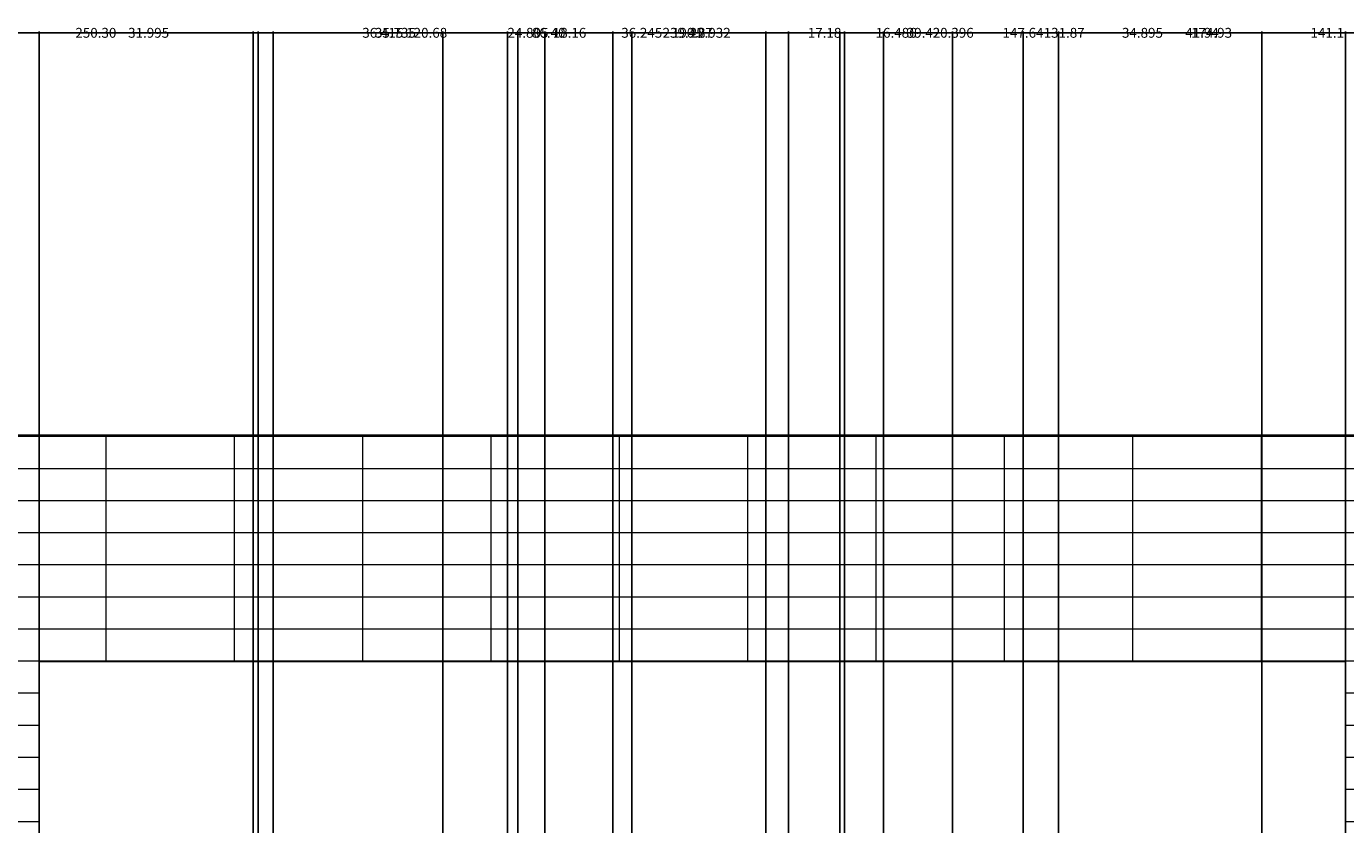
# Model space of a CAD drawing. Units: inches. Extents: x 241 to 943, y 109 to 1396.
# Tile 32 of 34: x 532 to 725, y 1279 to 1396. Entities that reach past the tile are written whole.
import ezdxf

# ---------------------------------------------------------------- set-up
doc = ezdxf.new("R2010")
doc.units = ezdxf.units.IN
doc.header["$MEASUREMENT"] = 0
for name, color, linetype, lineweight in [('A-ANNO-DIMS', 2, 'Continuous', 18), ('A-ELEV', 7, 'Continuous', 25), ('A-GLAZ', 4, 'Continuous', 18), ('A-WALL-PATT', 8, 'Continuous', 13)]:
    doc.layers.add(name, color=color, linetype=linetype, lineweight=lineweight)
doc.styles.get("Standard").update_dxf_attribs({"font": 'arial.ttf'})
doc.dimstyles.get("Standard").update_dxf_attribs({"dimtxt": 1.4375, "dimasz": 0.18, "dimexe": 0.18, "dimexo": 0.0625, "dimgap": 0.09, "dimtad": 0, "dimtih": 1, "dimtoh": 1, "dimdec": 4, "dimzin": 0, "dimdsep": 46, "dimlunit": 4, "dimtxsty": 'Standard', "dimcen": 0.09, "dimadec": 0, "dimazin": 0, "dimtfac": 1, "dimtdec": 4, "dimtofl": 0, "dimtmove": 0, "dimatfit": 3, "dimfxl": 1, "dimtolj": 1, "dimtzin": 0, "dimarcsym": 0})

# ---------------------------------------------------------------- blocks, each defined once
blk = doc.blocks.new('*D12')
at = {"layer": 'A-ANNO-DIMS', "color": 0, "lineweight": -2, "transparency": 16777216}
for p, q in [((530.23, 384.24), (530.23, 1395.05)), ((530.41, 1394.87), (587.56, 1394.87)), ((650.73, 1394.87), (593.58, 1394.87)), ((650.91, 384.24), (650.91, 1395.05))]:
    blk.add_line(p, q, dxfattribs=at)
at = {"layer": 'A-ANNO-DIMS', "color": 0, "transparency": 16777216}
for points in [[(530.41, 1394.9), (530.41, 1394.84), (530.23, 1394.87)], [(650.73, 1394.9), (650.73, 1394.84), (650.91, 1394.87)]]:
    blk.add_solid(points, dxfattribs=at)
at = {"layer": 'Defpoints', "color": 0, "transparency": 16777216}
for p in [(650.91, 1394.87), (530.23, 384.18), (650.91, 384.18)]:
    blk.add_point(p, dxfattribs=at)
at = {"layer": 'A-ANNO-DIMS', "color": 0, "transparency": 16777216, "insert": (590.57, 1394.87), "char_height": 1.438, "attachment_point": 5}
blk.add_mtext('\\A1;120.68', dxfattribs=at)
blk = doc.blocks.new('*D13')
at = {"layer": 'A-ANNO-DIMS', "color": 0, "lineweight": -2, "transparency": 16777216}
for p, q in [((650.91, 384.24), (650.91, 1395.05)), ((651.09, 1394.87), (656.14, 1394.87)), ((667.21, 1394.87), (662.16, 1394.87)), ((667.39, 290.06), (667.39, 1395.05))]:
    blk.add_line(p, q, dxfattribs=at)
at = {"layer": 'A-ANNO-DIMS', "color": 0, "transparency": 16777216}
for points in [[(651.09, 1394.9), (651.09, 1394.84), (650.91, 1394.87)], [(667.21, 1394.9), (667.21, 1394.84), (667.39, 1394.87)]]:
    blk.add_solid(points, dxfattribs=at)
at = {"layer": 'Defpoints', "color": 0, "transparency": 16777216}
for p in [(667.39, 1394.87), (650.91, 384.18), (667.39, 290)]:
    blk.add_point(p, dxfattribs=at)
at = {"layer": 'A-ANNO-DIMS', "color": 0, "transparency": 16777216, "insert": (659.15, 1394.87), "char_height": 1.438, "attachment_point": 5}
blk.add_mtext('\\A1;16.486', dxfattribs=at)
blk = doc.blocks.new('*D14')
at = {"layer": 'A-ANNO-DIMS', "color": 0, "lineweight": -2, "transparency": 16777216}
for p, q in [((667.39, 290.06), (667.39, 1395.05)), ((667.57, 1394.87), (727.7, 1394.87)), ((793.85, 1394.87), (733.72, 1394.87)), ((794.03, 290.06), (794.03, 1395.05))]:
    blk.add_line(p, q, dxfattribs=at)
at = {"layer": 'A-ANNO-DIMS', "color": 0, "transparency": 16777216}
for points in [[(667.57, 1394.9), (667.57, 1394.84), (667.39, 1394.87)], [(793.85, 1394.9), (793.85, 1394.84), (794.03, 1394.87)]]:
    blk.add_solid(points, dxfattribs=at)
at = {"layer": 'Defpoints', "color": 0, "transparency": 16777216}
for p in [(794.03, 1394.87), (667.39, 290), (794.03, 290)]:
    blk.add_point(p, dxfattribs=at)
at = {"layer": 'A-ANNO-DIMS', "color": 0, "transparency": 16777216, "insert": (730.71, 1394.87), "char_height": 1.438, "attachment_point": 5}
blk.add_mtext('\\A1;126.63', dxfattribs=at)
blk = doc.blocks.new('*D18')
at = {"layer": 'A-ANNO-DIMS', "color": 0, "lineweight": -2, "transparency": 16777216}
for p, q in [((508.31, 1336.18), (508.31, 1395.05)), ((508.49, 1394.87), (624.94, 1394.87)), ((747.58, 1394.87), (631.12, 1394.87)), ((747.76, 1336.18), (747.76, 1395.05))]:
    blk.add_line(p, q, dxfattribs=at)
at = {"layer": 'A-ANNO-DIMS', "color": 0, "transparency": 16777216}
for points in [[(508.49, 1394.9), (508.49, 1394.84), (508.31, 1394.87)], [(747.58, 1394.9), (747.58, 1394.84), (747.76, 1394.87)]]:
    blk.add_solid(points, dxfattribs=at)
at = {"layer": 'Defpoints', "color": 0, "transparency": 16777216}
for p in [(747.76, 1394.87), (508.31, 1336.12), (747.76, 1336.12)]:
    blk.add_point(p, dxfattribs=at)
at = {"layer": 'A-ANNO-DIMS', "color": 0, "transparency": 16777216, "insert": (628.03, 1394.87), "char_height": 1.438, "attachment_point": 5}
blk.add_mtext('\\A1;239.45', dxfattribs=at)
blk = doc.blocks.new('*D56')
at = {"layer": 'A-ANNO-DIMS', "color": 0, "lineweight": -2, "transparency": 16777216}
for p, q in [((533.95, 1303.09), (533.95, 1395.05)), ((534.13, 1394.87), (626.38, 1394.87)), ((724.64, 1394.87), (632.39, 1394.87)), ((724.82, 1303.09), (724.82, 1395.05))]:
    blk.add_line(p, q, dxfattribs=at)
at = {"layer": 'A-ANNO-DIMS', "color": 0, "transparency": 16777216}
for points in [[(534.13, 1394.9), (534.13, 1394.84), (533.95, 1394.87)], [(724.64, 1394.9), (724.64, 1394.84), (724.82, 1394.87)]]:
    blk.add_solid(points, dxfattribs=at)
at = {"layer": 'Defpoints', "color": 0, "transparency": 16777216}
for p in [(724.82, 1394.87), (533.95, 1303.03), (724.82, 1303.03)]:
    blk.add_point(p, dxfattribs=at)
at = {"layer": 'A-ANNO-DIMS', "color": 0, "transparency": 16777216, "insert": (629.39, 1394.87), "char_height": 1.438, "attachment_point": 5}
blk.add_mtext('\\A1;190.87', dxfattribs=at)
blk = doc.blocks.new('*D57')
at = {"layer": 'A-ANNO-DIMS', "color": 0, "lineweight": -2, "transparency": 16777216}
for p, q in [((508.31, 1070.92), (508.31, 1395.05)), ((508.49, 1394.87), (518.04, 1394.87)), ((533.77, 1394.87), (524.21, 1394.87)), ((533.95, 1108.23), (533.95, 1395.05))]:
    blk.add_line(p, q, dxfattribs=at)
at = {"layer": 'A-ANNO-DIMS', "color": 0, "transparency": 16777216}
for points in [[(508.49, 1394.9), (508.49, 1394.84), (508.31, 1394.87)], [(533.77, 1394.9), (533.77, 1394.84), (533.95, 1394.87)]]:
    blk.add_solid(points, dxfattribs=at)
at = {"layer": 'Defpoints', "color": 0, "transparency": 16777216}
for p in [(533.95, 1394.87), (533.95, 1108.17), (508.31, 1070.85)]:
    blk.add_point(p, dxfattribs=at)
at = {"layer": 'A-ANNO-DIMS', "color": 0, "transparency": 16777216, "insert": (521.13, 1394.87), "char_height": 1.438, "attachment_point": 5}
blk.add_mtext('\\A1;25.646', dxfattribs=at)
blk = doc.blocks.new('*D62')
at = {"layer": 'A-ANNO-DIMS', "color": 0, "lineweight": -2, "transparency": 16777216}
for p, q in [((424.11, 568.89), (424.11, 1395.05)), ((424.29, 1394.87), (492.35, 1394.87)), ((565.02, 1394.87), (496.96, 1394.87)), ((565.2, 568.89), (565.2, 1395.05))]:
    blk.add_line(p, q, dxfattribs=at)
at = {"layer": 'A-ANNO-DIMS', "color": 0, "transparency": 16777216}
for points in [[(424.29, 1394.9), (424.29, 1394.84), (424.11, 1394.87)], [(565.02, 1394.9), (565.02, 1394.84), (565.2, 1394.87)]]:
    blk.add_solid(points, dxfattribs=at)
at = {"layer": 'Defpoints', "color": 0, "transparency": 16777216}
for p in [(565.2, 1394.87), (424.11, 568.83), (565.2, 568.83)]:
    blk.add_point(p, dxfattribs=at)
at = {"layer": 'A-ANNO-DIMS', "color": 0, "transparency": 16777216, "insert": (494.66, 1394.87), "char_height": 1.438, "attachment_point": 5}
blk.add_mtext('\\A1;141.1', dxfattribs=at)
blk = doc.blocks.new('*D63')
at = {"layer": 'A-ANNO-DIMS', "color": 0, "lineweight": -2, "transparency": 16777216}
for p, q in [((651.6, 568.89), (651.6, 1395.05)), ((651.78, 1394.87), (719.84, 1394.87)), ((792.51, 1394.87), (724.45, 1394.87)), ((792.69, 568.89), (792.69, 1395.05))]:
    blk.add_line(p, q, dxfattribs=at)
at = {"layer": 'A-ANNO-DIMS', "color": 0, "transparency": 16777216}
for points in [[(651.78, 1394.9), (651.78, 1394.84), (651.6, 1394.87)], [(792.51, 1394.9), (792.51, 1394.84), (792.69, 1394.87)]]:
    blk.add_solid(points, dxfattribs=at)
at = {"layer": 'Defpoints', "color": 0, "transparency": 16777216}
for p in [(792.69, 1394.87), (651.6, 568.83), (792.69, 568.83)]:
    blk.add_point(p, dxfattribs=at)
at = {"layer": 'A-ANNO-DIMS', "color": 0, "transparency": 16777216, "insert": (722.14, 1394.87), "char_height": 1.438, "attachment_point": 5}
blk.add_mtext('\\A1;141.1', dxfattribs=at)
blk = doc.blocks.new('*D65')
at = {"layer": 'A-ANNO-DIMS', "color": 0, "lineweight": -2, "transparency": 16777216}
for p, q in [((424.11, 700.85), (424.11, 1395.05)), ((424.29, 1394.87), (505.52, 1394.87)), ((592.77, 1394.87), (511.54, 1394.87)), ((592.95, 700.85), (592.95, 1395.05))]:
    blk.add_line(p, q, dxfattribs=at)
at = {"layer": 'A-ANNO-DIMS', "color": 0, "transparency": 16777216}
for points in [[(424.29, 1394.9), (424.29, 1394.84), (424.11, 1394.87)], [(592.77, 1394.9), (592.77, 1394.84), (592.95, 1394.87)]]:
    blk.add_solid(points, dxfattribs=at)
at = {"layer": 'Defpoints', "color": 0, "transparency": 16777216}
for p in [(592.95, 1394.87), (424.11, 700.79), (592.95, 700.79)]:
    blk.add_point(p, dxfattribs=at)
at = {"layer": 'A-ANNO-DIMS', "color": 0, "transparency": 16777216, "insert": (508.53, 1394.87), "char_height": 1.438, "attachment_point": 5}
blk.add_mtext('\\A1;168.85', dxfattribs=at)
blk = doc.blocks.new('*D66')
at = {"layer": 'A-ANNO-DIMS', "color": 0, "lineweight": -2, "transparency": 16777216}
for p, q in [((617.76, 702.85), (617.76, 1395.05)), ((617.94, 1394.87), (680.69, 1394.87)), ((749.45, 1394.87), (686.7, 1394.87)), ((749.63, 702.85), (749.63, 1395.05))]:
    blk.add_line(p, q, dxfattribs=at)
at = {"layer": 'A-ANNO-DIMS', "color": 0, "transparency": 16777216}
for points in [[(617.94, 1394.9), (617.94, 1394.84), (617.76, 1394.87)], [(749.45, 1394.9), (749.45, 1394.84), (749.63, 1394.87)]]:
    blk.add_solid(points, dxfattribs=at)
at = {"layer": 'Defpoints', "color": 0, "transparency": 16777216}
for p in [(749.63, 1394.87), (617.76, 702.79), (749.63, 702.79)]:
    blk.add_point(p, dxfattribs=at)
at = {"layer": 'A-ANNO-DIMS', "color": 0, "transparency": 16777216, "insert": (683.7, 1394.87), "char_height": 1.438, "attachment_point": 5}
blk.add_mtext('\\A1;131.87', dxfattribs=at)
blk = doc.blocks.new('*D67')
at = {"layer": 'A-ANNO-DIMS', "color": 0, "lineweight": -2, "transparency": 16777216}
for p, q in [((389.04, 773.55), (389.04, 1395.05)), ((389.22, 1394.87), (495.34, 1394.87)), ((607.64, 1394.87), (501.52, 1394.87)), ((607.82, 773.55), (607.82, 1395.05))]:
    blk.add_line(p, q, dxfattribs=at)
at = {"layer": 'A-ANNO-DIMS', "color": 0, "transparency": 16777216}
for points in [[(389.22, 1394.9), (389.22, 1394.84), (389.04, 1394.87)], [(607.64, 1394.9), (607.64, 1394.84), (607.82, 1394.87)]]:
    blk.add_solid(points, dxfattribs=at)
at = {"layer": 'Defpoints', "color": 0, "transparency": 16777216}
for p in [(607.82, 1394.87), (389.04, 773.49), (607.82, 773.49)]:
    blk.add_point(p, dxfattribs=at)
at = {"layer": 'A-ANNO-DIMS', "color": 0, "transparency": 16777216, "insert": (498.43, 1394.87), "char_height": 1.438, "attachment_point": 5}
blk.add_mtext('\\A1;218.77', dxfattribs=at)
blk = doc.blocks.new('*D68')
at = {"layer": 'A-ANNO-DIMS', "color": 0, "lineweight": -2, "transparency": 16777216}
for p, q in [((617.76, 841.6), (617.76, 1395.05)), ((617.94, 1394.87), (702.22, 1394.87)), ((792.51, 1394.87), (708.23, 1394.87)), ((792.69, 841.6), (792.69, 1395.05))]:
    blk.add_line(p, q, dxfattribs=at)
at = {"layer": 'A-ANNO-DIMS', "color": 0, "transparency": 16777216}
for points in [[(617.94, 1394.9), (617.94, 1394.84), (617.76, 1394.87)], [(792.51, 1394.9), (792.51, 1394.84), (792.69, 1394.87)]]:
    blk.add_solid(points, dxfattribs=at)
at = {"layer": 'Defpoints', "color": 0, "transparency": 16777216}
for p in [(792.69, 1394.87), (617.76, 841.54), (792.69, 841.54)]:
    blk.add_point(p, dxfattribs=at)
at = {"layer": 'A-ANNO-DIMS', "color": 0, "transparency": 16777216, "insert": (705.23, 1394.87), "char_height": 1.438, "attachment_point": 5}
blk.add_mtext('\\A1;174.93', dxfattribs=at)
blk = doc.blocks.new('*D69')
at = {"layer": 'A-ANNO-DIMS', "color": 0, "lineweight": -2, "transparency": 16777216}
for p, q in [((389.04, 941.55), (389.04, 1395.05)), ((389.22, 1394.87), (476.28, 1394.87)), ((567.95, 1394.87), (480.9, 1394.87)), ((568.13, 941.55), (568.13, 1395.05))]:
    blk.add_line(p, q, dxfattribs=at)
at = {"layer": 'A-ANNO-DIMS', "color": 0, "transparency": 16777216}
for points in [[(389.22, 1394.9), (389.22, 1394.84), (389.04, 1394.87)], [(567.95, 1394.9), (567.95, 1394.84), (568.13, 1394.87)]]:
    blk.add_solid(points, dxfattribs=at)
at = {"layer": 'Defpoints', "color": 0, "transparency": 16777216}
for p in [(568.13, 1394.87), (389.04, 941.49), (568.13, 941.49)]:
    blk.add_point(p, dxfattribs=at)
at = {"layer": 'A-ANNO-DIMS', "color": 0, "transparency": 16777216, "insert": (478.59, 1394.87), "char_height": 1.438, "attachment_point": 5}
blk.add_mtext('\\A1;179.1', dxfattribs=at)
blk = doc.blocks.new('*D70')
at = {"layer": 'A-ANNO-DIMS', "color": 0, "lineweight": -2, "transparency": 16777216}
for p, q in [((603.87, 1009.6), (603.87, 1395.05)), ((604.05, 1394.87), (674.69, 1394.87)), ((751.33, 1394.87), (680.69, 1394.87)), ((751.51, 1009.6), (751.51, 1395.05))]:
    blk.add_line(p, q, dxfattribs=at)
at = {"layer": 'A-ANNO-DIMS', "color": 0, "transparency": 16777216}
for points in [[(604.05, 1394.9), (604.05, 1394.84), (603.87, 1394.87)], [(751.33, 1394.9), (751.33, 1394.84), (751.51, 1394.87)]]:
    blk.add_solid(points, dxfattribs=at)
at = {"layer": 'Defpoints', "color": 0, "transparency": 16777216}
for p in [(751.51, 1394.87), (603.87, 1009.54), (751.51, 1009.54)]:
    blk.add_point(p, dxfattribs=at)
at = {"layer": 'A-ANNO-DIMS', "color": 0, "transparency": 16777216, "insert": (677.69, 1394.87), "char_height": 1.438, "attachment_point": 5}
blk.add_mtext('\\A1;147.64', dxfattribs=at)
blk = doc.blocks.new('*D82')
at = {"layer": 'A-ANNO-DIMS', "color": 0, "lineweight": -2, "transparency": 16777216}
for p, q in [((565.2, 568.89), (565.2, 1395.05)), ((565.38, 1394.87), (605.89, 1394.87)), ((651.42, 1394.87), (610.91, 1394.87)), ((651.6, 568.89), (651.6, 1395.05))]:
    blk.add_line(p, q, dxfattribs=at)
at = {"layer": 'A-ANNO-DIMS', "color": 0, "transparency": 16777216}
for points in [[(565.38, 1394.9), (565.38, 1394.84), (565.2, 1394.87)], [(651.42, 1394.9), (651.42, 1394.84), (651.6, 1394.87)]]:
    blk.add_solid(points, dxfattribs=at)
at = {"layer": 'Defpoints', "color": 0, "transparency": 16777216}
for p in [(651.6, 1394.87), (565.2, 568.83), (651.6, 568.83)]:
    blk.add_point(p, dxfattribs=at)
at = {"layer": 'A-ANNO-DIMS', "color": 0, "transparency": 16777216, "insert": (608.4, 1394.87), "char_height": 1.438, "attachment_point": 5}
blk.add_mtext('\\A1;86.40', dxfattribs=at)
blk = doc.blocks.new('*D83')
at = {"layer": 'A-ANNO-DIMS', "color": 0, "lineweight": -2, "transparency": 16777216}
for p, q in [((592.95, 700.85), (592.95, 1395.05)), ((593.13, 1394.87), (602.27, 1394.87)), ((617.58, 1394.87), (608.45, 1394.87)), ((617.76, 702.85), (617.76, 1395.05))]:
    blk.add_line(p, q, dxfattribs=at)
at = {"layer": 'A-ANNO-DIMS', "color": 0, "transparency": 16777216}
for points in [[(593.13, 1394.9), (593.13, 1394.84), (592.95, 1394.87)], [(617.58, 1394.9), (617.58, 1394.84), (617.76, 1394.87)]]:
    blk.add_solid(points, dxfattribs=at)
at = {"layer": 'Defpoints', "color": 0, "transparency": 16777216}
for p in [(617.76, 1394.87), (617.76, 702.79), (592.95, 700.79)]:
    blk.add_point(p, dxfattribs=at)
at = {"layer": 'A-ANNO-DIMS', "color": 0, "transparency": 16777216, "insert": (605.36, 1394.87), "char_height": 1.438, "attachment_point": 5}
blk.add_mtext('\\A1;24.805', dxfattribs=at)
blk = doc.blocks.new('*D89')
at = {"layer": 'A-ANNO-DIMS', "color": 0, "lineweight": -2, "transparency": 16777216}
for p, q in [((377.04, 841.6), (377.04, 1395.05)), ((377.22, 1394.87), (494.32, 1394.87)), ((617.58, 1394.87), (500.48, 1394.87)), ((617.76, 841.6), (617.76, 1395.05))]:
    blk.add_line(p, q, dxfattribs=at)
at = {"layer": 'A-ANNO-DIMS', "color": 0, "transparency": 16777216}
for points in [[(377.22, 1394.9), (377.22, 1394.84), (377.04, 1394.87)], [(617.58, 1394.9), (617.58, 1394.84), (617.76, 1394.87)]]:
    blk.add_solid(points, dxfattribs=at)
at = {"layer": 'Defpoints', "color": 0, "transparency": 16777216}
for p in [(617.76, 1394.87), (377.04, 841.54), (617.76, 841.54)]:
    blk.add_point(p, dxfattribs=at)
at = {"layer": 'A-ANNO-DIMS', "color": 0, "transparency": 16777216, "insert": (497.4, 1394.87), "char_height": 1.438, "attachment_point": 5}
blk.add_mtext('\\A1;240.72', dxfattribs=at)
blk = doc.blocks.new('*D90')
at = {"layer": 'A-ANNO-DIMS', "color": 0, "lineweight": -2, "transparency": 16777216}
for p, q in [((568.13, 941.55), (568.13, 1395.05)), ((568.31, 1394.87), (582.92, 1394.87)), ((603.69, 1394.87), (589.08, 1394.87)), ((603.87, 902.92), (603.87, 1395.05))]:
    blk.add_line(p, q, dxfattribs=at)
at = {"layer": 'A-ANNO-DIMS', "color": 0, "transparency": 16777216}
for points in [[(568.31, 1394.9), (568.31, 1394.84), (568.13, 1394.87)], [(603.69, 1394.9), (603.69, 1394.84), (603.87, 1394.87)]]:
    blk.add_solid(points, dxfattribs=at)
at = {"layer": 'Defpoints', "color": 0, "transparency": 16777216}
for p in [(603.87, 1394.87), (568.13, 941.49), (603.87, 902.85)]:
    blk.add_point(p, dxfattribs=at)
at = {"layer": 'A-ANNO-DIMS', "color": 0, "transparency": 16777216, "insert": (586, 1394.87), "char_height": 1.438, "attachment_point": 5}
blk.add_mtext('\\A1;35.735', dxfattribs=at)
blk = doc.blocks.new('*D99')
at = {"layer": 'A-ANNO-DIMS', "color": 0, "lineweight": -2, "transparency": 16777216}
for p, q in [((417.09, 181.71), (417.09, 1395.05)), ((417.27, 1394.87), (539.16, 1394.87)), ((667.21, 1394.87), (545.33, 1394.87)), ((667.39, 214.58), (667.39, 1395.05))]:
    blk.add_line(p, q, dxfattribs=at)
at = {"layer": 'A-ANNO-DIMS', "color": 0, "transparency": 16777216}
for points in [[(417.27, 1394.9), (417.27, 1394.84), (417.09, 1394.87)], [(667.21, 1394.9), (667.21, 1394.84), (667.39, 1394.87)]]:
    blk.add_solid(points, dxfattribs=at)
at = {"layer": 'Defpoints', "color": 0, "transparency": 16777216}
for p in [(667.39, 1394.87), (667.39, 214.52), (417.09, 181.65)]:
    blk.add_point(p, dxfattribs=at)
at = {"layer": 'A-ANNO-DIMS', "color": 0, "transparency": 16777216, "insert": (542.24, 1394.87), "char_height": 1.438, "attachment_point": 5}
blk.add_mtext('\\A1;250.30', dxfattribs=at)
blk = doc.blocks.new('*D104')
at = {"layer": 'A-ANNO-DIMS', "color": 0, "lineweight": -2, "transparency": 16777216}
for p, q in [((533.95, 1108.23), (533.95, 1395.05)), ((534.13, 1394.87), (546.87, 1394.87)), ((565.77, 1394.87), (553.03, 1394.87)), ((565.95, 1110.23), (565.95, 1395.05))]:
    blk.add_line(p, q, dxfattribs=at)
at = {"layer": 'A-ANNO-DIMS', "color": 0, "transparency": 16777216}
for points in [[(534.13, 1394.9), (534.13, 1394.84), (533.95, 1394.87)], [(565.77, 1394.9), (565.77, 1394.84), (565.95, 1394.87)]]:
    blk.add_solid(points, dxfattribs=at)
at = {"layer": 'Defpoints', "color": 0, "transparency": 16777216}
for p in [(565.95, 1394.87), (565.95, 1110.17), (533.95, 1108.17)]:
    blk.add_point(p, dxfattribs=at)
at = {"layer": 'A-ANNO-DIMS', "color": 0, "transparency": 16777216, "insert": (549.95, 1394.87), "char_height": 1.438, "attachment_point": 5}
blk.add_mtext('\\A1;31.995', dxfattribs=at)
blk = doc.blocks.new('*D105')
at = {"layer": 'A-ANNO-DIMS', "color": 0, "lineweight": -2, "transparency": 16777216}
for p, q in [((565.95, 1110.23), (565.95, 1395.05)), ((566.13, 1394.87), (581.08, 1394.87)), ((602.18, 1394.87), (587.23, 1394.87)), ((602.36, 1110.23), (602.36, 1395.05))]:
    blk.add_line(p, q, dxfattribs=at)
at = {"layer": 'A-ANNO-DIMS', "color": 0, "transparency": 16777216}
for points in [[(566.13, 1394.9), (566.13, 1394.84), (565.95, 1394.87)], [(602.18, 1394.9), (602.18, 1394.84), (602.36, 1394.87)]]:
    blk.add_solid(points, dxfattribs=at)
at = {"layer": 'Defpoints', "color": 0, "transparency": 16777216}
for p in [(602.36, 1394.87), (565.95, 1110.17), (602.36, 1110.17)]:
    blk.add_point(p, dxfattribs=at)
at = {"layer": 'A-ANNO-DIMS', "color": 0, "transparency": 16777216, "insert": (584.15, 1394.87), "char_height": 1.438, "attachment_point": 5}
blk.add_mtext('\\A1;36.415', dxfattribs=at)
blk = doc.blocks.new('*D106')
at = {"layer": 'A-ANNO-DIMS', "color": 0, "lineweight": -2, "transparency": 16777216}
for p, q in [((602.36, 1110.23), (602.36, 1395.05)), ((602.54, 1394.87), (608.99, 1394.87)), ((620.34, 1394.87), (613.89, 1394.87)), ((620.52, 1110.23), (620.52, 1395.05))]:
    blk.add_line(p, q, dxfattribs=at)
at = {"layer": 'A-ANNO-DIMS', "color": 0, "transparency": 16777216}
for points in [[(602.54, 1394.9), (602.54, 1394.84), (602.36, 1394.87)], [(620.34, 1394.9), (620.34, 1394.84), (620.52, 1394.87)]]:
    blk.add_solid(points, dxfattribs=at)
at = {"layer": 'Defpoints', "color": 0, "transparency": 16777216}
for p in [(620.52, 1394.87), (602.36, 1110.17), (620.52, 1110.17)]:
    blk.add_point(p, dxfattribs=at)
at = {"layer": 'A-ANNO-DIMS', "color": 0, "transparency": 16777216, "insert": (611.44, 1394.87), "char_height": 1.438, "attachment_point": 5}
blk.add_mtext('\\A1;18.16', dxfattribs=at)
blk = doc.blocks.new('*D107')
at = {"layer": 'A-ANNO-DIMS', "color": 0, "lineweight": -2, "transparency": 16777216}
for p, q in [((620.52, 1110.23), (620.52, 1395.05)), ((620.7, 1394.87), (628.91, 1394.87)), ((643.27, 1394.87), (635.07, 1394.87)), ((643.45, 1110.23), (643.45, 1395.05))]:
    blk.add_line(p, q, dxfattribs=at)
at = {"layer": 'A-ANNO-DIMS', "color": 0, "transparency": 16777216}
for points in [[(620.7, 1394.9), (620.7, 1394.84), (620.52, 1394.87)], [(643.27, 1394.9), (643.27, 1394.84), (643.45, 1394.87)]]:
    blk.add_solid(points, dxfattribs=at)
at = {"layer": 'Defpoints', "color": 0, "transparency": 16777216}
for p in [(643.45, 1394.87), (620.52, 1110.17), (643.45, 1110.17)]:
    blk.add_point(p, dxfattribs=at)
at = {"layer": 'A-ANNO-DIMS', "color": 0, "transparency": 16777216, "insert": (631.99, 1394.87), "char_height": 1.438, "attachment_point": 5}
blk.add_mtext('\\A1;22.932', dxfattribs=at)
blk = doc.blocks.new('*D108')
at = {"layer": 'A-ANNO-DIMS', "color": 0, "lineweight": -2, "transparency": 16777216}
for p, q in [((643.45, 1110.23), (643.45, 1395.05)), ((643.63, 1394.87), (660.66, 1394.87)), ((682.69, 1394.87), (665.67, 1394.87)), ((682.87, 1110.23), (682.87, 1395.05))]:
    blk.add_line(p, q, dxfattribs=at)
at = {"layer": 'A-ANNO-DIMS', "color": 0, "transparency": 16777216}
for points in [[(643.63, 1394.9), (643.63, 1394.84), (643.45, 1394.87)], [(682.69, 1394.9), (682.69, 1394.84), (682.87, 1394.87)]]:
    blk.add_solid(points, dxfattribs=at)
at = {"layer": 'Defpoints', "color": 0, "transparency": 16777216}
for p in [(682.87, 1394.87), (643.45, 1110.17), (682.87, 1110.17)]:
    blk.add_point(p, dxfattribs=at)
at = {"layer": 'A-ANNO-DIMS', "color": 0, "transparency": 16777216, "insert": (663.16, 1394.87), "char_height": 1.438, "attachment_point": 5}
blk.add_mtext('\\A1;39.42', dxfattribs=at)
blk = doc.blocks.new('*D109')
at = {"layer": 'A-ANNO-DIMS', "color": 0, "lineweight": -2, "transparency": 16777216}
for p, q in [((682.87, 1110.23), (682.87, 1395.05)), ((683.05, 1394.87), (701.31, 1394.87)), ((724.64, 1394.87), (706.39, 1394.87)), ((724.82, 1108.23), (724.82, 1395.05))]:
    blk.add_line(p, q, dxfattribs=at)
at = {"layer": 'A-ANNO-DIMS', "color": 0, "transparency": 16777216}
for points in [[(683.05, 1394.9), (683.05, 1394.84), (682.87, 1394.87)], [(724.64, 1394.9), (724.64, 1394.84), (724.82, 1394.87)]]:
    blk.add_solid(points, dxfattribs=at)
at = {"layer": 'Defpoints', "color": 0, "transparency": 16777216}
for p in [(724.82, 1394.87), (682.87, 1110.17), (724.82, 1108.17)]:
    blk.add_point(p, dxfattribs=at)
at = {"layer": 'A-ANNO-DIMS', "color": 0, "transparency": 16777216, "insert": (703.85, 1394.87), "char_height": 1.438, "attachment_point": 5}
blk.add_mtext('\\A1;41.94', dxfattribs=at)
blk = doc.blocks.new('*D113')
at = {"layer": 'A-ANNO-DIMS', "color": 0, "lineweight": -2, "transparency": 16777216}
for p, q in [((603.87, 902.92), (603.87, 1395.05)), ((604.05, 1394.87), (618.91, 1394.87)), ((639.93, 1394.87), (625.07, 1394.87)), ((640.11, 902.92), (640.11, 1395.05))]:
    blk.add_line(p, q, dxfattribs=at)
at = {"layer": 'A-ANNO-DIMS', "color": 0, "transparency": 16777216}
for points in [[(604.05, 1394.9), (604.05, 1394.84), (603.87, 1394.87)], [(639.93, 1394.9), (639.93, 1394.84), (640.11, 1394.87)]]:
    blk.add_solid(points, dxfattribs=at)
at = {"layer": 'Defpoints', "color": 0, "transparency": 16777216}
for p in [(640.11, 1394.87), (603.87, 902.85), (640.11, 902.85)]:
    blk.add_point(p, dxfattribs=at)
at = {"layer": 'A-ANNO-DIMS', "color": 0, "transparency": 16777216, "insert": (621.99, 1394.87), "char_height": 1.438, "attachment_point": 5}
blk.add_mtext('\\A1;36.245', dxfattribs=at)
blk = doc.blocks.new('*D114')
at = {"layer": 'A-ANNO-DIMS', "color": 0, "lineweight": -2, "transparency": 16777216}
for p, q in [((640.11, 902.92), (640.11, 1395.05)), ((640.29, 1394.87), (646.25, 1394.87)), ((657.11, 1394.87), (651.15, 1394.87)), ((657.29, 902.92), (657.29, 1395.05))]:
    blk.add_line(p, q, dxfattribs=at)
at = {"layer": 'A-ANNO-DIMS', "color": 0, "transparency": 16777216}
for points in [[(640.29, 1394.9), (640.29, 1394.84), (640.11, 1394.87)], [(657.11, 1394.9), (657.11, 1394.84), (657.29, 1394.87)]]:
    blk.add_solid(points, dxfattribs=at)
at = {"layer": 'Defpoints', "color": 0, "transparency": 16777216}
for p in [(657.29, 1394.87), (640.11, 902.85), (657.29, 902.85)]:
    blk.add_point(p, dxfattribs=at)
at = {"layer": 'A-ANNO-DIMS', "color": 0, "transparency": 16777216, "insert": (648.7, 1394.87), "char_height": 1.438, "attachment_point": 5}
blk.add_mtext('\\A1;17.18', dxfattribs=at)
blk = doc.blocks.new('*D115')
at = {"layer": 'A-ANNO-DIMS', "color": 0, "lineweight": -2, "transparency": 16777216}
for p, q in [((657.29, 902.92), (657.29, 1395.05)), ((657.47, 1394.87), (664.4, 1394.87)), ((677.51, 1394.87), (670.58, 1394.87)), ((677.69, 902.92), (677.69, 1395.05))]:
    blk.add_line(p, q, dxfattribs=at)
at = {"layer": 'A-ANNO-DIMS', "color": 0, "transparency": 16777216}
for points in [[(657.47, 1394.9), (657.47, 1394.84), (657.29, 1394.87)], [(677.51, 1394.9), (677.51, 1394.84), (677.69, 1394.87)]]:
    blk.add_solid(points, dxfattribs=at)
at = {"layer": 'Defpoints', "color": 0, "transparency": 16777216}
for p in [(677.69, 1394.87), (657.29, 902.85), (677.69, 902.85)]:
    blk.add_point(p, dxfattribs=at)
at = {"layer": 'A-ANNO-DIMS', "color": 0, "transparency": 16777216, "insert": (667.49, 1394.87), "char_height": 1.438, "attachment_point": 5}
blk.add_mtext('\\A1;20.396', dxfattribs=at)
blk = doc.blocks.new('*D116')
at = {"layer": 'A-ANNO-DIMS', "color": 0, "lineweight": -2, "transparency": 16777216}
for p, q in [((677.69, 902.92), (677.69, 1395.05)), ((677.87, 1394.87), (692.06, 1394.87)), ((712.4, 1394.87), (698.22, 1394.87)), ((712.58, 902.92), (712.58, 1395.05))]:
    blk.add_line(p, q, dxfattribs=at)
at = {"layer": 'A-ANNO-DIMS', "color": 0, "transparency": 16777216}
for points in [[(677.87, 1394.9), (677.87, 1394.84), (677.69, 1394.87)], [(712.4, 1394.9), (712.4, 1394.84), (712.58, 1394.87)]]:
    blk.add_solid(points, dxfattribs=at)
at = {"layer": 'Defpoints', "color": 0, "transparency": 16777216}
for p in [(712.58, 1394.87), (677.69, 902.85), (712.58, 902.85)]:
    blk.add_point(p, dxfattribs=at)
at = {"layer": 'A-ANNO-DIMS', "color": 0, "transparency": 16777216, "insert": (695.14, 1394.87), "char_height": 1.438, "attachment_point": 5}
blk.add_mtext('\\A1;34.895', dxfattribs=at)
blk = doc.blocks.new('*D117')
at = {"layer": 'A-ANNO-DIMS', "color": 0, "lineweight": -2, "transparency": 16777216}
for p, q in [((712.58, 902.92), (712.58, 1395.05)), ((712.76, 1394.87), (729.54, 1394.87)), ((751.33, 1394.87), (734.55, 1394.87)), ((751.51, 902.92), (751.51, 1395.05))]:
    blk.add_line(p, q, dxfattribs=at)
at = {"layer": 'A-ANNO-DIMS', "color": 0, "transparency": 16777216}
for points in [[(712.76, 1394.9), (712.76, 1394.84), (712.58, 1394.87)], [(751.33, 1394.9), (751.33, 1394.84), (751.51, 1394.87)]]:
    blk.add_solid(points, dxfattribs=at)
at = {"layer": 'Defpoints', "color": 0, "transparency": 16777216}
for p in [(751.51, 1394.87), (712.58, 902.85), (751.51, 902.85)]:
    blk.add_point(p, dxfattribs=at)
at = {"layer": 'A-ANNO-DIMS', "color": 0, "transparency": 16777216, "insert": (732.05, 1394.87), "char_height": 1.438, "attachment_point": 5}
blk.add_mtext('\\A1;38.92', dxfattribs=at)

msp = doc.modelspace()

# ---------------------------------------------------------------- hatches: boundary and pattern name
at = {"layer": 'A-WALL-PATT'}
h = msp.add_hatch(dxfattribs=at)
h.set_pattern_fill('GRATE', color=256, scale=150)
h.paths.add_polyline_path([(747.7579, 1238.8538), (747.7579, 1275.9142), (747.7579, 1336.1154), (508.3064, 1336.1154), (508.3064, 1275.9142), (508.3064, 1238.8538), (508.3064, 1177.5382), (508.3064, 1109.4916), (508.3064, 1070.8538), (553.5166, 1070.8538), (749.6328, 1070.8538)])
h.paths.add_polyline_path([(533.952, 1108.1686), (533.952, 1177.7336), (533.952, 1303.0286), (724.819, 1303.0286), (724.819, 1108.1686)], flags=16)
h.paths.add_polyline_path([(535.952, 1110.1686), (535.952, 1175.7336), (722.819, 1175.7336), (722.819, 1110.1686)], flags=0)
h.paths.add_polyline_path([(643.4534, 1134.0739), (622.521, 1134.0739), (622.521, 1136.0739), (643.4534, 1136.0739)], flags=0)
h.paths.add_polyline_path([(617.7594, 568.8295), (617.7594, 734.8538), (377.0391, 734.8538), (377.0391, 566.8538), (377.0391, 400.8295), (417.0913, 400.8295), (618.9643, 400.8295)])
h.paths.add_polyline_path([(424.1086, 496.4395), (424.1086, 568.8295), (565.2023, 568.8295), (565.2023, 496.4395)], flags=16)
h.paths.add_polyline_path([(426.1086, 498.4395), (426.1086, 566.8295), (563.2023, 566.8295), (563.2023, 508.9074), (563.2023, 498.4395)], flags=0)
h.paths.add_polyline_path([(508.0803, 508.9074), (508.0803, 519.3754), (450.9259, 519.3754), (450.9259, 525.3816), (445.5808, 525.3816, -1), (445.5808, 527.3816), (450.9259, 527.3816), (450.9259, 566.8295), (508.0803, 566.8295), (537.4269, 566.8295), (537.4269, 508.9074)], flags=0)
h.paths.add_polyline_path([(506.0803, 521.3754), (452.9259, 521.3754), (452.9259, 564.8295), (506.0803, 564.8295)], flags=0)
h.paths.add_polyline_path([(424.1086, 628.4013), (424.1086, 700.7912), (592.9542, 700.7912), (592.9542, 628.4013)], flags=16)
h.paths.add_polyline_path([(426.1086, 630.4013), (426.1086, 698.7912), (590.8792, 698.7912), (590.8792, 630.4013)], flags=0)
h.paths.add_polyline_path([(508.1906, 651.3371), (508.0803, 651.3371), (450.9259, 651.3371), (428.0291, 651.3371), (428.0291, 698.7912), (451.9767, 698.7912), (508.0803, 698.7912), (537.4269, 698.7912), (563.2023, 698.7912), (563.2023, 659.3434), (563.9297, 659.3434), (563.9297, 651.3371)], flags=0)
h.paths.add_polyline_path([(506.0803, 653.3371), (452.9259, 653.3371), (452.9259, 657.3434), (445.5808, 657.3434, -1), (445.5808, 659.3434), (452.9259, 659.3434), (452.9259, 696.7912), (506.0803, 696.7912)], flags=0)

# ---------------------------------------------------------------- linework, layer by layer
at = {"layer": 'A-ELEV'}
msp.add_line((747.7579, 1336.1154), (508.3064, 1336.1154), dxfattribs=at)
at = {"layer": 'A-GLAZ'}
msp.add_lwpolyline([(533.952, 1303.0286), (724.819, 1303.0286), (724.819, 1108.1686), (533.952, 1108.1686)], close=True, dxfattribs=at)

# ---------------------------------------------------------------- dimensions: what is measured, and where the dimension line sits
at = {"layer": 'A-ANNO-DIMS'}
for base, p1, p2, override, picture, middle in [((617.7594, 1394.8654), (377.0391, 841.5382), (617.7594, 841.5382), {"dimdec": 2, "dimlfac": 1, "dimrnd": 0, "dimzin": 0, "dimdsep": 46, "dimlunit": 2}, '*D89', (497.3993, 1394.8654)), ((607.8162, 1394.8654), (389.0429, 773.4916), (607.8162, 773.4916), {"dimdec": 2, "dimlfac": 1, "dimrnd": 0, "dimzin": 0, "dimdsep": 46, "dimlunit": 2}, '*D67', (498.4295, 1394.8654)), ((568.1348, 1394.8654), (389.0429, 941.4916), (568.1348, 941.4916), {"dimdec": 1, "dimlfac": 1, "dimrnd": 0, "dimzin": 0, "dimdsep": 46, "dimlunit": 2}, '*D69', (478.5888, 1394.8654)), ((667.3935, 1394.8654), (417.0913, 181.649), (667.3935, 214.5189), {"dimdec": 2, "dimlfac": 1, "dimrnd": 0, "dimzin": 0, "dimdsep": 46, "dimlunit": 2}, '*D99', (542.2424, 1394.8654)), ((565.2023, 1394.8654), (424.1086, 568.8295), (565.2023, 568.8295), {"dimdec": 1, "dimlfac": 1, "dimrnd": 0, "dimzin": 0, "dimdsep": 46, "dimlunit": 2}, '*D62', (494.6554, 1394.8654)), ((592.9542, 1394.8654), (424.1086, 700.7912), (592.9542, 700.7912), {"dimdec": 2, "dimlfac": 1, "dimrnd": 0, "dimzin": 0, "dimdsep": 46, "dimlunit": 2}, '*D65', (508.5314, 1394.8654)), ((747.7579, 1394.8654), (508.3064, 1336.1154), (747.7579, 1336.1154), {"dimdec": 2, "dimlfac": 1, "dimrnd": 0, "dimzin": 0, "dimdsep": 46, "dimlunit": 2}, '*D18', (628.0322, 1394.8654)), ((533.952, 1394.8654), (508.3064, 1070.8538), (533.952, 1108.1686), {"dimdec": 3, "dimlfac": 1, "dimrnd": 0, "dimzin": 0, "dimdsep": 46, "dimlunit": 2}, '*D57', (521.1292, 1394.8654)), ((650.907, 1394.8654), (530.2303, 384.1784), (650.907, 384.1784), {"dimdec": 2, "dimlfac": 1, "dimrnd": 0, "dimzin": 0, "dimdsep": 46, "dimlunit": 2}, '*D12', (590.5686, 1394.8654)), ((724.819, 1394.8654), (533.952, 1303.0286), (724.819, 1303.0286), {"dimdec": 2, "dimlfac": 1, "dimrnd": 0, "dimzin": 0, "dimdsep": 46, "dimlunit": 2}, '*D56', (629.3855, 1394.8654)), ((565.947, 1394.8654), (533.952, 1108.1686), (565.947, 1110.1686), {"dimdec": 3, "dimlfac": 1, "dimrnd": 0, "dimzin": 0, "dimdsep": 46, "dimlunit": 2}, '*D104', (549.9495, 1394.8654)), ((651.5974, 1394.8654), (565.2023, 568.8295), (651.5974, 568.8295), {"dimdec": 2, "dimlfac": 1, "dimrnd": 0, "dimzin": 0, "dimdsep": 46, "dimlunit": 2}, '*D82', (608.3998, 1394.8654)), ((602.3616, 1394.8654), (565.947, 1110.1686), (602.3616, 1110.1686), {"dimdec": 3, "dimlfac": 1, "dimrnd": 0, "dimzin": 0, "dimdsep": 46, "dimlunit": 2}, '*D105', (584.1543, 1394.8654)), ((603.8694, 1394.8654), (568.1348, 941.4916), (603.8694, 902.8538), {"dimdec": 3, "dimlfac": 1, "dimrnd": 0, "dimzin": 0, "dimdsep": 46, "dimlunit": 2}, '*D90', (586.0021, 1394.8654)), ((617.7594, 1394.8654), (592.9542, 700.7912), (617.7594, 702.7912), {"dimdec": 3, "dimlfac": 1, "dimrnd": 0, "dimzin": 0, "dimdsep": 46, "dimlunit": 2}, '*D83', (605.3568, 1394.8654)), ((620.521, 1394.8654), (602.3616, 1110.1686), (620.521, 1110.1686), {"dimdec": 2, "dimlfac": 1, "dimrnd": 0, "dimzin": 0, "dimdsep": 46, "dimlunit": 2}, '*D106', (611.4413, 1394.8654)), ((751.5078, 1394.8654), (603.8694, 1009.5382), (751.5078, 1009.5382), {"dimdec": 2, "dimlfac": 1, "dimrnd": 0, "dimzin": 0, "dimdsep": 46, "dimlunit": 2}, '*D70', (677.6886, 1394.8654)), ((640.1141, 1394.8654), (603.8694, 902.8538), (640.1141, 902.8538), {"dimdec": 3, "dimlfac": 1, "dimrnd": 0, "dimzin": 0, "dimdsep": 46, "dimlunit": 2}, '*D113', (621.9918, 1394.8654)), ((749.6328, 1394.8654), (617.7594, 702.7912), (749.6328, 702.7912), {"dimdec": 2, "dimlfac": 1, "dimrnd": 0, "dimzin": 0, "dimdsep": 46, "dimlunit": 2}, '*D66', (683.6961, 1394.8654)), ((792.691, 1394.8654), (617.7594, 841.5382), (792.691, 841.5382), {"dimdec": 2, "dimlfac": 1, "dimrnd": 0, "dimzin": 0, "dimdsep": 46, "dimlunit": 2}, '*D68', (705.2252, 1394.8654)), ((643.4534, 1394.8654), (620.521, 1110.1686), (643.4534, 1110.1686), {"dimdec": 3, "dimlfac": 1, "dimrnd": 0, "dimzin": 0, "dimdsep": 46, "dimlunit": 2}, '*D107', (631.9872, 1394.8654)), ((657.2925, 1394.8654), (640.1141, 902.8538), (657.2925, 902.8538), {"dimdec": 2, "dimlfac": 1, "dimrnd": 0, "dimzin": 0, "dimdsep": 46, "dimlunit": 2}, '*D114', (648.7033, 1394.8654)), ((682.8748, 1394.8654), (643.4534, 1110.1686), (682.8748, 1110.1686), {"dimdec": 2, "dimlfac": 1, "dimrnd": 0, "dimzin": 0, "dimdsep": 46, "dimlunit": 2}, '*D108', (663.1641, 1394.8654)), ((667.39345, 1394.86544), (650.90697, 384.17836), (667.39345, 289.99842), {"dimdec": 3, "dimlfac": 1, "dimrnd": 0, "dimzin": 0, "dimdsep": 46, "dimlunit": 2}, '*D13', (659.15021, 1394.86544)), ((792.691, 1394.8654), (651.5974, 568.8295), (792.691, 568.8295), {"dimdec": 1, "dimlfac": 1, "dimrnd": 0, "dimzin": 0, "dimdsep": 46, "dimlunit": 2}, '*D63', (722.1442, 1394.8654)), ((677.6886, 1394.8654), (657.2925, 902.8538), (677.6886, 902.8538), {"dimdec": 3, "dimlfac": 1, "dimrnd": 0, "dimzin": 0, "dimdsep": 46, "dimlunit": 2}, '*D115', (667.4905, 1394.8654)), ((794.0275, 1394.8654), (667.3935, 289.9984), (794.0275, 289.9984), {"dimdec": 2, "dimlfac": 1, "dimrnd": 0, "dimzin": 0, "dimdsep": 46, "dimlunit": 2}, '*D14', (730.7105, 1394.8654)), ((712.5839, 1394.8654), (677.6886, 902.8538), (712.5839, 902.8538), {"dimdec": 3, "dimlfac": 1, "dimrnd": 0, "dimzin": 0, "dimdsep": 46, "dimlunit": 2}, '*D116', (695.1363, 1394.8654)), ((724.819, 1394.8654), (682.8748, 1110.1686), (724.819, 1108.1686), {"dimdec": 2, "dimlfac": 1, "dimrnd": 0, "dimzin": 0, "dimdsep": 46, "dimlunit": 2}, '*D109', (703.8469, 1394.8654)), ((751.5078, 1394.8654), (712.5839, 902.8538), (751.5078, 902.8538), {"dimdec": 2, "dimlfac": 1, "dimrnd": 0, "dimzin": 0, "dimdsep": 46, "dimlunit": 2}, '*D117', (732.0459, 1394.8654))]:
    dim = msp.add_linear_dim(base=base, p1=p1, p2=p2, dimstyle='Standard', override=override, dxfattribs=at)
    dim.commit()
    dim.dimension.update_dxf_attribs({"geometry": picture, "text_midpoint": middle})

doc.saveas('drawing.dxf')
